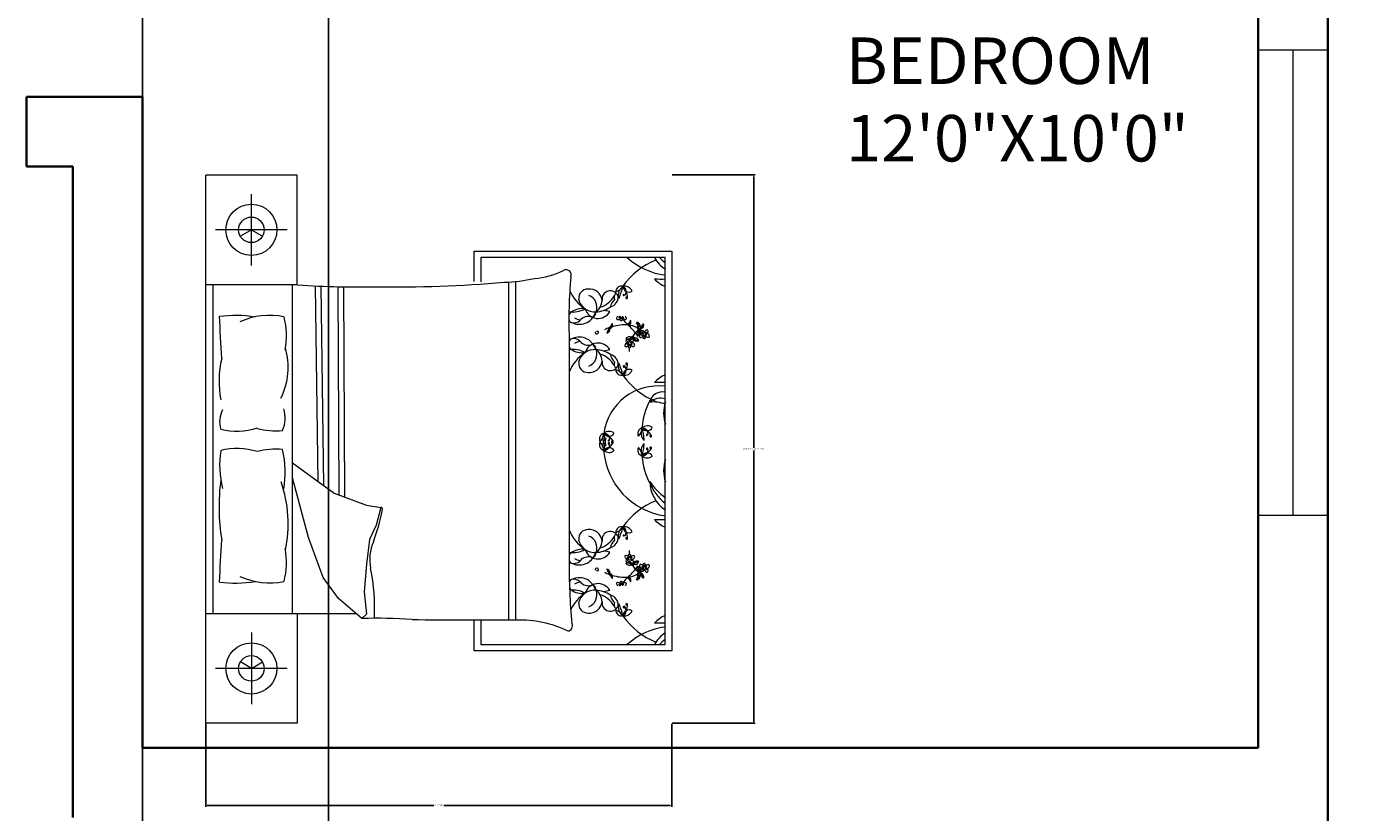
# Model space of a CAD drawing. Units: inches. Extents: x -43 to 1296, y -568 to 542.
# Tile 10 of 14: x 1016 to 1187, y -354 to -253. Entities that reach past the tile are written whole.
import ezdxf

# ---------------------------------------------------------------- set-up
doc = ezdxf.new("R2010")
doc.units = ezdxf.units.IN
doc.header["$MEASUREMENT"] = 0
for name, color, linetype, lineweight in [('A-ANNO-DIMS', 2, 'Continuous', 18), ('A-AREA-IDEN', 7, 'Continuous', 18), ('A-FURN', 8, 'Continuous', 13), ('A-GLAZ', 6, 'Continuous', 18), ('A-WALL', 7, 'Continuous', 35)]:
    doc.layers.add(name, color=color, linetype=linetype, lineweight=lineweight)
doc.styles.get("Standard").update_dxf_attribs({"font": 'arial.ttf'})
doc.dimstyles.get("Standard").update_dxf_attribs({"dimtxt": 0.18, "dimasz": 0.18, "dimexe": 0.18, "dimexo": 0.0625, "dimgap": 0.09, "dimtad": 0, "dimtih": 1, "dimtoh": 1, "dimdec": 0, "dimzin": 0, "dimdsep": 46, "dimlunit": 3, "dimtxsty": 'Standard', "dimcen": 0.09, "dimadec": 0, "dimazin": 0, "dimtfac": 1, "dimtdec": 0, "dimtofl": 0, "dimtmove": 0, "dimatfit": 3, "dimfxl": 1, "dimtolj": 1, "dimtzin": 0, "dimarcsym": 0})

# ---------------------------------------------------------------- blocks, each defined once
blk = doc.blocks.new('*D4')
at = {"layer": 'A-ANNO-DIMS', "color": 0, "lineweight": -2, "transparency": 16777216}
for p, q in [((1184.19, -3.76), (1201.25, -3.76)), ((1201.07, -3.94), (1201.07, -240.61)), ((1201.07, -483.58), (1201.07, -246.91)), ((1184.19, -483.76), (1201.25, -483.76))]:
    blk.add_line(p, q, dxfattribs=at)
at = {"layer": 'A-ANNO-DIMS', "color": 0, "transparency": 16777216}
for points in [[(1201.04, -3.94), (1201.1, -3.94), (1201.07, -3.76)], [(1201.04, -483.58), (1201.1, -483.58), (1201.07, -483.76)]]:
    blk.add_solid(points, dxfattribs=at)
at = {"layer": 'Defpoints', "color": 0, "transparency": 16777216}
for p in [(1184.13, -3.76), (1184.13, -483.76), (1201.07, -483.76)]:
    blk.add_point(p, dxfattribs=at)
at = {"layer": 'A-ANNO-DIMS', "color": 0, "transparency": 16777216, "insert": (1201.07, -243.76), "char_height": 6, "attachment_point": 5}
blk.add_mtext("\\A1;40'", dxfattribs=at)
blk = doc.blocks.new('BED-SUITE-71')
for p, q in [((0, 0), (0, 70.73)), ((5.89, 59.04), (5.89, 68.28)), ((10.52, 63.66), (1.27, 63.66)), ((34.67, 56.98), (34.67, 60.9)), ((34.67, 60.9), (60.15, 60.9)), ((35.49, 60.08), (35.49, 56.97)), ((59.33, 60.08), (35.49, 60.08)), ((59.33, 10.16), (59.33, 60.08)), ((60.15, 60.9), (60.15, 9.34)), ((0.91, 56.59), (0.91, 14.15)), ((11.18, 14.15), (11.18, 56.59)), ((14.12, 56.4), (14.47, 31.21)), ((39.09, 56.91), (39.09, 13.33)), ((39.97, 56.97), (39.97, 13.33)), ((14.84, 56.37), (15.21, 30.69)), ((17.07, 56.33), (17.18, 29.47)), ((17.8, 56.34), (17.91, 29.2)), ((52.16, 53.11), (51.36, 53.27)), ((46.92, 49.73), (46.92, 21.01)), ((52.16, 48.17), (51.36, 48.01)), ((11.18, 33.58), (16.57, 29.7)), ((13.28, 23.97), (11.18, 31.68)), ((16.57, 29.7), (20.73, 28.13)), ((20.73, 28.13), (22.59, 27.84)), ((22.59, 27.84), (22.01, 25.55)), ((15.14, 18.81), (13.28, 23.97)), ((22.01, 25.55), (21.15, 23.69)), ((21.15, 23.69), (20.73, 20.53)), ((52.16, 22.07), (51.36, 22.23)), ((20.73, 20.53), (20.44, 16.95)), ((17.15, 16.09), (15.14, 18.81)), ((52.16, 17.13), (51.36, 16.97)), ((20.15, 13.51), (17.15, 16.09)), ((20.44, 16.95), (20.73, 14.09)), ((0, 14.15), (19.41, 14.15)), ((20.73, 14.09), (20.15, 13.51)), ((34.67, 9.34), (34.67, 13.34)), ((35.49, 13.34), (35.49, 10.16)), ((5.89, 11.69), (5.89, 2.45)), ((60.15, 9.34), (34.67, 9.34)), ((35.49, 10.16), (59.33, 10.16)), ((10.52, 7.07), (1.27, 7.07))]:
    blk.add_line(p, q)
for points in [[(0, 56.59), (11.79, 56.59), (11.79, 70.73), (0, 70.73)], [(5.89, 63.66), (4.47, 62.83)], [(5.89, 63.66), (7.32, 62.83)], [(11.79, 14.15), (11.79, 0), (0, 0)], [(5.89, 7.07), (4.47, 7.9)], [(5.89, 7.07), (7.32, 7.9)]]:
    blk.add_lwpolyline(points)
for points in [[(38.53, 56.89, 0.056112), (42.42, 57.4, 0.095341), (46.17, 58.4)], [(1.76, 52.52, -0.074897), (6.38, 52.44, 0.472817)], [(6.64, 38.06, -0.14099), (1.93, 37.91, -0.235245)], [(6.64, 35.04, 0.14099), (1.93, 35.18, 0.235245)], [(1.76, 18.21, 0.074897), (6.38, 18.3, -0.472817)], [(26.63, 13.37, 0.001242), (40.05, 13.33, -0.127202), (46.74, 11.91)]]:
    blk.add_lwpolyline(points, format="xyb")
for centre, radius in [((5.89, 63.66), 3.3), ((5.89, 63.66), 1.65), ((56.62, 50.21), 0.18), ((54.73, 49.03), 0.18), ((54.73, 21.21), 0.18), ((56.62, 20.03), 0.18), ((5.89, 7.07), 3.3), ((5.89, 7.07), 1.65)]:
    blk.add_circle(centre, radius)
for centre, radius, start, end in [((60.58, 66.96), 9.24, 228.1144, 262.255), ((61.82, 62.33), 4.5, 209.8884, 236.5383), ((62.65, 63.95), 5.61, 223.5186, 233.6964), ((46.53, 57.86), 0.645, 336.5219, 123.8264), ((61.49, 51.16), 9.24, 111.4092, 145.6135), ((19.82, 183.39), 127.09, 266.1, 270.9282), ((24.44, 222.08), 165.79, 269.1145, 274.8735), ((115.71, 51.89), 68.83, 175.2402, 181.8035), ((53.69, 55.63), 0.766, 76.272, 177.0484), ((52.52, 57.2), 1.58, 284.7031, 328.6173), ((54.72, 55.19), 1.46, 125.7657, 194.5347), ((47.56, 57.77), 6.46, 332.8176, 347.4827), ((54.09, 55.37), 1.02, 20.9613, 102.2885), ((54.64, 56.4), 0.771, 181.7131, 301.5367), ((52.11, 54.84), 2.34, 2.0648, 41.1598), ((53.52, 55.71), 0.756, 316.2238, 62.3173), ((60.77, 59.81), 3.76, 221.0454, 247.4453), ((58.76, 70.09), 12.78, 266.3481, 272.5919), ((51.9, 57.95), 5.35, 203.6453, 236.3329), ((49.33, 54.83), 1.19, 88.9462, 185.5144), ((50.21, 55.2), 2.13, 193.079, 274.7067), ((49.5, 54.34), 1.69, 7.1143, 95.0551), ((48.86, 53.68), 1.64, 338.5779, 68.4181), ((49.88, 56.84), 3.34, 288.2955, 328.7386), ((52.22, 54.73), 1.06, 19.1312, 189.736), ((51.9, 54.99), 1.33, 285.6955, 4.031), ((53.66, 53.56), 1.41, 128.4175, 173.8338), ((53.37, 54.95), 0.651, 126.7319, 206.0245), ((53.95, 55.26), 0.0602, 20.2667, 316.2271), ((54.27, 54.93), 0.0557, 52.0591, 168.5166), ((54.33, 54.92), 0.115, 168.5166, 2.0648), ((47.44, 55.99), 2.93, 259.249, 301.1782), ((47.7, 52.36), 0.852, 127.675, 162.5814), ((48.2, 53.72), 2.25, 240.8249, 340.7178), ((48.71, 50.78), 2.73, 85.2696, 124.215), ((50.64, 53.99), 1.76, 196.8663, 330.0915), ((49.9, 52.88), 0.439, 254.8529, 12.6959), ((48.71, 50.78), 2.73, 53.6555, 57.2989), ((49.12, 54.64), 2.05, 305.9599, 357.6409), ((50.15, 56.87), 3.8, 273.4924, 303.7117), ((-671.38, 13.54), 674.27, 2.85022, 3.31479), ((8.24, 43.51), 9.12, 78.2417, 114.8684), ((0.94, 50), 9.48, 348.9631, 14.8961), ((47.7, 52.36), 0.852, 196.6343, 225.5483), ((47.53, 52.72), 1.06, 246.1646, 318.4347), ((48.61, 54.06), 2.03, 240.0851, 262.564), ((49.41, 51.05), 1.45, 74.8529, 138.4347), ((52.16, 51.3), 0.339, 265.7131, 351.6568), ((51.42, 52), 1.14, 313.6929, 321.7899), ((52.67, 51.22), 0.371, 115.5379, 168.6744), ((51.41, 51.75), 1.12, 329.344, 349.7412), ((54.13, 45.54), 5.86, 86.1723, 106.4158), ((50.52, 51.5), 1.99, 352.8698, 1.6736), ((53.16, 52.22), 0.139, 125.0752, 284.7644), ((53.38, 52.27), 0.3, 127.3642, 168.4363), ((53.14, 52.51), 0.433, 277.4968, 341.2737), ((53.48, 52.31), 0.172, 88.1325, 178.8919), ((53.83, 52.13), 0.372, 136.3462, 189.6513), ((53.62, 52.09), 0.155, 189.6513, 312.3208), ((53.66, 52.52), 0.18, 183.2768, 356.7232), ((54.22, 52.2), 0.59, 164.2829, 186.9148), ((53.52, 52.19), 0.295, 312.3208, 40.2111), ((54.15, 52.53), 0.419, 201.6382, 274.947), ((53.59, 51.95), 0.547, 42.3896, 66.5724), ((59.11, 56.28), 6.72, 217.9541, 226.8459), ((53.99, 52.27), 0.297, 10.9597, 52.2379), ((54.17, 52.25), 0.138, 274.947, 37.5263), ((54.64, 51.46), 0.144, 112.5583, 214.2343), ((54.54, 51.72), 0.339, 265.7131, 351.6568), ((54.24, 51.91), 0.593, 297.3659, 329.344), ((54.27, 48.45), 2.94, 60.7959, 85.244), ((48.02, 44.23), 9.66, 37.8256, 47.7588), ((53.8, 52.42), 1.14, 313.6929, 321.7899), ((55.05, 51.64), 0.371, 115.5379, 168.6744), ((53.79, 52.18), 1.12, 329.344, 349.7412), ((52.9, 51.92), 1.99, 352.8698, 1.6736), ((55.7, 51.52), 0.201, 33.0979, 123.1364), ((51.27, 48.68), 5.26, 31.1156, 34.8118), ((55.41, 51.17), 0.545, 2.3172, 70.5201), ((55.6, 51.29), 0.208, 315.7354, 31.1156), ((55.62, 51.23), 0.469, 352.6008, 57.1845), ((56.07, 51.34), 0.469, 252.8042, 349.6943), ((56.12, 51.38), 0.208, 248.2452, 323.6254), ((55.93, 51.5), 0.545, 291.7087, 3.0299), ((52.05, 54.37), 5.26, 323.6254, 327.3216), ((56.36, 51.37), 0.201, 325.6077, 55.6462), ((48.2, 47.57), 2.25, 19.2822, 119.1751), ((47.53, 48.57), 1.06, 41.5653, 113.8354), ((50.48, 50.45), 0.222, 169.5864, 349.5616), ((50.57, 50.44), 0.136, 349.5616, 167.2949), ((54.13, 45.54), 5.86, 110.1059, 116.9968), ((52.16, 50.36), 0.371, 129.5056, 182.6421), ((51.09, 51.22), 1.12, 308.4388, 328.836), ((50.9, 52.13), 1.99, 296.5064, 305.3102), ((50.88, 51.11), 1.14, 336.3901, 344.4871), ((52.12, 50.82), 0.144, 83.9457, 185.6216), ((51.54, 50.95), 0.593, 328.836, 0.8141), ((51.85, 50.78), 0.339, 306.5232, 32.4668), ((52.26, 51.04), 0.144, 112.5583, 214.2343), ((51.86, 51.49), 0.593, 297.3659, 329.344), ((54.46, 50.41), 0.821, 253.6301, 325.4631), ((54.69, 49.27), 0.581, 82.0748, 142.6895), ((54.62, 50.06), 0.597, 228.342, 274.9894), ((54.64, 49.97), 0.499, 273.8774, 357.1501), ((55.27, 49.07), 0.568, 121.9501, 165.2442), ((54.84, 50.32), 0.483, 262.0748, 308.2393), ((58.17, 48.15), 3.52, 156.1523, 156.9499), ((55.06, 49.41), 0.178, 44.3732, 121.9501), ((55.61, 49.82), 0.499, 181.4625, 249.4747), ((55.53, 50.22), 0.483, 215.1128, 261.2773), ((55.92, 50.19), 0.821, 197.889, 269.722), ((58.17, 48.15), 3.52, 130.182, 149.456), ((55.37, 49.17), 0.581, 20.6625, 81.2773), ((56.23, 50.16), 0.581, 139.3812, 199.9959), ((55.15, 50.58), 0.821, 310.9365, 22.7695), ((55.53, 50.53), 0.597, 285.6484, 332.2957), ((55.86, 51.04), 0.157, 135.7354, 318.1297), ((55.43, 50.85), 0.483, 319.3812, 5.5456), ((55.98, 51.04), 0.157, 68.2452, 250.6395), ((57.29, 48.08), 3.14, 111.7087, 116.2181), ((54.27, 48.45), 2.94, 47.5083, 55.9967), ((55.62, 50.5), 0.499, 331.1838, 51.6792), ((56.13, 49.9), 0.139, 125.0752, 284.7644), ((56.35, 49.96), 0.3, 93.635, 168.4363), ((56.31, 50.43), 0.176, 138.2946, 276.2474), ((56.11, 50.2), 0.433, 277.4968, 341.2737), ((56.37, 50.4), 0.246, 358.5719, 143.8954), ((56.45, 50), 0.172, 88.1325, 178.8919), ((56.52, 50.6), 0.248, 208.8493, 269.9355), ((56.31, 50.54), 0.283, 274.2123, 318.1587), ((56.8, 49.81), 0.372, 136.3462, 189.6513), ((56.59, 49.78), 0.155, 189.6513, 312.3208), ((57.19, 49.88), 0.59, 164.2829, 186.9148), ((57.17, 50.25), 0.568, 121.9501, 165.2442), ((56.49, 49.88), 0.295, 312.3208, 40.2111), ((57.12, 50.21), 0.419, 201.6382, 274.947), ((56.78, 50.47), 0.119, 262.868, 7.094), ((56.56, 49.64), 0.547, 42.3896, 66.5724), ((56.76, 50.57), 0.355, 278.5614, 22.5914), ((56.96, 49.96), 0.297, 10.9597, 118.7804), ((56.96, 50.58), 0.178, 44.3732, 121.9501), ((57.14, 49.93), 0.138, 274.947, 37.5263), ((1.63, 45.91), 9, 333.8761, 16.1746), ((47.7, 48.93), 0.852, 134.4517, 156.7144), ((47.7, 48.93), 0.852, 203.2856, 232.325), ((47.44, 45.3), 2.93, 58.8218, 100.2867), ((48.71, 50.51), 2.73, 235.785, 274.7304), ((48.61, 47.23), 2.03, 97.436, 119.9149), ((50.21, 46.08), 2.13, 85.2933, 166.921), ((49.41, 50.23), 1.45, 221.5653, 285.1471), ((50.64, 47.29), 1.76, 29.9085, 163.1337), ((48.86, 47.61), 1.64, 291.5819, 21.4221), ((49.9, 48.41), 0.439, 347.3041, 105.1471), ((48.71, 50.51), 2.73, 302.7011, 306.3445), ((49.12, 46.65), 2.05, 2.3591, 54.0401), ((50.15, 44.42), 3.8, 56.2883, 86.5076), ((54.23, 48.72), 0.139, 125.0752, 284.7644), ((54.45, 48.78), 0.3, 93.635, 168.4363), ((54.41, 49.25), 0.176, 138.2946, 276.2474), ((54.21, 49.02), 0.433, 277.4968, 341.2737), ((54.48, 49.23), 0.246, 358.5719, 143.8954), ((54.56, 48.82), 0.172, 88.1325, 178.8919), ((54.62, 49.42), 0.248, 208.8493, 269.9355), ((54.41, 49.36), 0.283, 274.2123, 318.1587), ((54.9, 48.63), 0.372, 136.3462, 189.6513), ((54.69, 48.6), 0.155, 189.6513, 312.3208), ((58.17, 48.15), 3.52, 175.2415, 182.8929), ((55.29, 48.7), 0.59, 164.2829, 186.9148), ((54.59, 48.7), 0.295, 312.3208, 40.2111), ((55.22, 49.03), 0.419, 201.6382, 274.947), ((54.88, 49.29), 0.119, 262.868, 7.094), ((54.66, 48.46), 0.547, 42.3896, 66.5724), ((54.86, 49.39), 0.355, 278.5614, 22.5914), ((55.06, 48.78), 0.297, 10.9597, 118.7804), ((55.24, 48.75), 0.138, 274.947, 37.5263), ((55.66, 49.91), 0.597, 248.3627, 295.0101), ((14.14, 44.13), 12.43, 166.3427, 191.1841), ((51.9, 43.33), 5.35, 123.6671, 158.5059), ((49.33, 46.45), 1.19, 174.4856, 271.0538), ((49.5, 46.94), 1.69, 264.9449, 352.8857), ((49.88, 44.45), 3.34, 31.2614, 71.7045), ((52.22, 46.55), 1.06, 170.264, 340.8688), ((53.66, 47.73), 1.41, 186.1662, 231.5825), ((51.9, 46.3), 1.33, 355.969, 74.3045), ((53.37, 46.33), 0.651, 153.9755, 233.2681), ((54.72, 46.09), 1.46, 165.4653, 234.2343), ((47.56, 43.51), 6.46, 12.5173, 27.1824), ((52.11, 46.45), 2.34, 318.8402, 357.9352), ((53.99, 46.03), 0.0999, 43.7762, 339.7183), ((54.33, 46.37), 0.115, 357.9352, 191.4834), ((54.27, 46.35), 0.0557, 191.4834, 307.9409), ((53.69, 45.65), 0.766, 182.9516, 283.728), ((52.52, 44.09), 1.58, 31.3827, 75.2969), ((53.52, 45.58), 0.756, 297.6827, 43.7762), ((54.64, 44.89), 0.771, 58.4633, 178.2869), ((54.09, 45.91), 1.02, 257.7115, 339.0387), ((61.49, 50.13), 9.24, 214.3865, 248.5908), ((60.77, 41.48), 3.76, 112.5547, 138.9546), ((58.45, 36.38), 7.15, 82.8636, 171.8197), ((58.94, 41.1), 1.66, 76.3898, 169.0739), ((58.76, 31.19), 12.78, 87.4081, 93.6519), ((65.53, 37.39), 9.24, 152.5854, 175.5377), ((58.72, 39.85), 2.1, 72.8609, 131.9049), ((57.79, 37.31), 4.14, 68.117, 96.6195), ((64.19, 39.97), 5.08, 162.9798, 196.4569), ((5.29, 38.88), 3.5, 153.3437, 196.1026), ((6.51, 39.36), 3.75, 335.0183, 18.5407), ((9.01, 46.39), 8.67, 254.1707, 275.9871), ((52.06, 36.64), 1.02, 50.8855, 132.2127), ((56.53, 37.37), 0.766, 106.1963, 206.9726), ((54.74, 38.15), 1.58, 314.6273, 358.5415), ((57.65, 37.51), 1.46, 155.6899, 224.4589), ((57.01, 37.35), 1.02, 50.8855, 132.2127), ((56.97, 38.51), 0.771, 211.6373, 331.4609), ((55.56, 35.9), 2.34, 31.989, 71.0841), ((50.15, 36.17), 6.46, 2.7418, 17.407), ((56.35, 37.35), 0.756, 346.148, 92.2415), ((66.81, 37.96), 7.51, 174.3643, 175.6213), ((71.95, 34), 13.42, 160.0972, 160.2783), ((51.58, 36.66), 0.766, 106.1963, 206.9726), ((51.58, 35.93), 0.766, 153.0274, 253.8037), ((49.79, 37.44), 1.58, 314.6273, 358.5415), ((49.79, 35.16), 1.58, 1.4585, 45.3727), ((52.7, 36.8), 1.46, 155.6899, 224.4589), ((52.7, 35.8), 1.46, 135.5411, 204.3101), ((52.03, 37.8), 0.771, 211.6373, 331.4609), ((51.4, 36.64), 0.756, 346.148, 92.2415), ((50.61, 35.19), 2.34, 31.989, 71.0841), ((45.2, 35.47), 6.46, 2.7418, 17.407), ((45.2, 37.13), 6.46, 342.593, 357.2582), ((50.61, 37.41), 2.34, 288.9159, 328.011), ((51.4, 35.95), 0.756, 267.7585, 13.852), ((52, 36.48), 0.0602, 50.1909, 346.0209), ((52.04, 36.11), 0.0999, 13.852, 309.9245), ((52.5, 36.37), 0.115, 198.4408, 31.989), ((52.44, 36.35), 0.0557, 81.9833, 198.4408), ((52.5, 36.23), 0.115, 328.011, 161.5592), ((52.44, 36.25), 0.0557, 161.5592, 278.0167), ((57.65, 35.09), 1.46, 135.5411, 204.3101), ((50.15, 36.42), 6.46, 342.593, 357.2582), ((56.94, 37.19), 0.0602, 50.1909, 346.0209), ((57.39, 37.05), 0.0557, 81.9833, 198.4408), ((57.44, 37.07), 0.115, 198.4408, 31.989), ((14.39, 33.32), 12.6, 171.5249, 193.96), ((9.01, 26.7), 8.67, 84.0129, 105.8293), ((-2.21, 32.38), 12.47, 349.8617, 13.6238), ((52.03, 34.79), 0.771, 28.5391, 148.3627), ((52.06, 35.96), 1.02, 227.7873, 309.1145), ((60.58, 35.92), 9.24, 184.4623, 262.255), ((56.53, 35.23), 0.766, 153.0274, 253.8037), ((54.74, 34.45), 1.58, 1.4585, 45.3727), ((55.56, 36.7), 2.34, 288.9159, 328.011), ((56.35, 35.25), 0.756, 267.7585, 13.852), ((56.97, 34.09), 0.771, 28.5391, 148.3627), ((57.01, 35.25), 1.02, 227.7873, 309.1145), ((65.53, 35.21), 9.24, 184.4623, 207.4146), ((56.98, 35.4), 0.0999, 13.852, 309.9245), ((57.39, 35.54), 0.0557, 161.5592, 278.0167), ((57.44, 35.52), 0.115, 328.011, 161.5592), ((64.19, 32.63), 5.08, 163.5431, 197.0202), ((66.81, 34.64), 7.51, 184.3787, 185.6357), ((71.95, 38.59), 13.42, 199.7217, 199.9028), ((27.36, 27.9), 25.65, 172.2196, 189.497), ((-5.8, 25.72), 16.44, 348.0397, 19.2615), ((61.82, 31.28), 4.5, 181.272, 236.5383), ((64.23, 35.85), 8.34, 214.0123, 234.053), ((62.65, 32.9), 5.61, 197.8504, 233.6964), ((-4.14, 32.75), 27.43, 340.1194, 349.3383), ((22.64, 27.68), 0.171, 358.8623, 109.7536), ((61.49, 20.11), 9.24, 111.4092, 145.6135), ((58.76, 39.05), 12.78, 266.3481, 272.5919), ((60.77, 28.76), 3.76, 221.0454, 247.4453), ((51.9, 26.91), 5.35, 201.4941, 236.3329), ((49.33, 23.79), 1.19, 88.9462, 185.5144), ((49.5, 23.3), 1.69, 7.1143, 95.0551), ((48.86, 22.63), 1.64, 338.5779, 68.4181), ((49.88, 25.79), 3.34, 288.2955, 328.7386), ((52.22, 23.69), 1.06, 19.1312, 189.736), ((51.9, 23.94), 1.33, 285.6955, 4.031), ((53.37, 23.91), 0.651, 126.7319, 206.0245), ((53.69, 24.59), 0.766, 76.272, 177.0484), ((52.52, 26.15), 1.58, 284.7031, 328.6173), ((54.72, 24.15), 1.46, 125.7657, 194.5347), ((47.56, 26.73), 6.46, 332.8176, 347.4827), ((54.09, 24.33), 1.02, 20.9613, 102.2885), ((53.52, 24.66), 0.756, 316.2238, 62.3173), ((52.11, 23.79), 2.34, 2.0648, 41.1598), ((54.64, 25.35), 0.771, 181.7131, 301.5367), ((53.95, 24.22), 0.0602, 20.2667, 316.2271), ((54.27, 23.88), 0.0557, 52.0591, 168.5166), ((-671.38, 57.2), 674.27, 356.68521, 357.14978), ((0.94, 20.73), 9.48, 345.1039, 11.0369), ((26.92, 21.1), 5.76, 156.2616, 191.3392), ((47.44, 24.94), 2.93, 259.7133, 301.1782), ((48.71, 19.73), 2.73, 85.2696, 124.215), ((50.21, 24.15), 2.13, 193.079, 274.7067), ((50.64, 22.95), 1.76, 196.8663, 330.0915), ((49.12, 23.59), 2.05, 305.9599, 357.6409), ((50.15, 25.82), 3.8, 273.4924, 303.7117), ((53.66, 22.51), 1.41, 128.4175, 173.8338), ((54.33, 23.87), 0.115, 168.5166, 2.0648), ((58.17, 22.09), 3.52, 177.1071, 184.7585), ((120.54, 20.16), 73.63, 179.3433, 185.6887), ((47.7, 21.31), 0.852, 127.675, 156.7144), ((47.7, 21.31), 0.852, 203.229, 225.5483), ((48.2, 22.67), 2.25, 240.8249, 340.7178), ((47.53, 21.67), 1.06, 246.1646, 318.4347), ((48.61, 23.01), 2.03, 240.0851, 262.564), ((49.41, 20.01), 1.45, 74.8529, 138.4347), ((49.9, 21.83), 0.439, 254.8529, 12.6959), ((48.71, 19.73), 2.73, 53.6555, 57.2989), ((54.23, 21.52), 0.139, 75.2356, 234.9248), ((54.45, 21.46), 0.3, 191.5637, 266.365), ((54.41, 20.99), 0.176, 83.7526, 221.7054), ((54.62, 20.18), 0.597, 85.0106, 131.658), ((54.46, 19.83), 0.821, 34.5369, 106.3699), ((54.69, 20.97), 0.581, 217.3105, 277.9252), ((54.21, 21.22), 0.433, 18.7263, 82.5032), ((54.48, 21.01), 0.246, 216.1046, 1.4281), ((54.56, 21.42), 0.172, 181.1081, 271.8675), ((54.62, 20.82), 0.248, 90.0645, 151.1507), ((54.41, 20.88), 0.283, 41.8413, 85.7877), ((54.69, 21.64), 0.155, 47.6792, 170.3487), ((54.9, 21.61), 0.372, 170.3487, 223.6538), ((54.64, 20.27), 0.499, 2.8499, 86.1226), ((55.29, 21.53), 0.59, 173.0852, 195.7171), ((55.27, 21.16), 0.568, 194.7558, 238.0499), ((54.59, 21.54), 0.295, 319.7889, 47.6792), ((55.22, 21.21), 0.419, 85.053, 158.3618), ((54.88, 20.95), 0.119, 352.906, 97.132), ((54.66, 21.78), 0.547, 293.4276, 317.6104), ((55.06, 21.46), 0.297, 241.2196, 349.0403), ((54.86, 20.85), 0.355, 337.4086, 81.4386), ((58.17, 22.09), 3.52, 203.0501, 203.8477), ((55.06, 20.83), 0.178, 238.0499, 315.6268), ((55.61, 20.41), 0.499, 110.5253, 178.5375), ((55.92, 20.05), 0.821, 90.278, 162.111), ((55.53, 20.02), 0.483, 98.7227, 144.8872), ((55.24, 21.49), 0.138, 322.4737, 85.053), ((55.66, 20.33), 0.597, 64.9899, 111.6373), ((55.37, 21.07), 0.581, 278.7227, 339.3375), ((56.59, 20.46), 0.155, 47.6792, 170.3487), ((56.49, 20.36), 0.295, 319.7889, 47.6792), ((8.24, 27.22), 9.12, 245.1316, 281.7583), ((-4.9, 14.72), 26.7, 357.4519, 11.3392), ((50.48, 19.79), 0.222, 10.4384, 190.4136), ((50.57, 19.8), 0.136, 192.7051, 10.4384), ((54.13, 24.7), 5.86, 243.0032, 249.8941), ((51.09, 19.02), 1.12, 31.164, 51.5612), ((52.16, 19.88), 0.371, 177.3579, 230.4944), ((50.9, 18.11), 1.99, 54.6898, 63.4936), ((50.88, 19.13), 1.14, 15.5129, 23.6099), ((52.12, 19.42), 0.144, 174.3784, 276.0543), ((51.85, 19.46), 0.339, 327.5332, 53.4768), ((51.54, 19.29), 0.593, 359.1859, 31.164), ((52.26, 19.2), 0.144, 145.7657, 247.4417), ((52.16, 18.94), 0.339, 8.3432, 94.2869), ((51.86, 18.75), 0.593, 30.656, 62.6341), ((51.42, 18.24), 1.14, 38.2101, 46.3071), ((52.67, 19.02), 0.371, 191.3256, 244.4621), ((51.41, 18.49), 1.12, 10.2588, 30.656), ((54.13, 24.7), 5.86, 253.5842, 273.8277), ((50.52, 18.74), 1.99, 358.3264, 7.1302), ((59.11, 13.96), 6.72, 133.1541, 142.0459), ((54.64, 18.78), 0.144, 145.7657, 247.4417), ((48.02, 26.01), 9.66, 312.2412, 322.1744), ((54.27, 21.79), 2.94, 274.756, 299.2041), ((54.54, 18.52), 0.339, 8.3432, 94.2869), ((54.24, 18.33), 0.593, 30.656, 62.6341), ((54.84, 19.92), 0.483, 51.7607, 97.9252), ((58.17, 22.09), 3.52, 210.544, 229.818), ((55.41, 19.07), 0.545, 289.4799, 357.6828), ((51.27, 21.56), 5.26, 325.1882, 328.8844), ((56.23, 20.08), 0.581, 160.0041, 220.6188), ((55.15, 19.66), 0.821, 337.2305, 49.0635), ((55.53, 19.71), 0.597, 27.7043, 74.3516), ((55.86, 19.2), 0.157, 41.8703, 224.2646), ((55.6, 18.95), 0.208, 328.8844, 44.2646), ((55.43, 19.39), 0.483, 354.4544, 40.6188), ((55.98, 19.2), 0.157, 109.3605, 291.7548), ((55.62, 19.01), 0.469, 302.8155, 7.3992), ((57.29, 22.16), 3.14, 243.7819, 248.2913), ((54.27, 21.79), 2.94, 304.0033, 312.4917), ((55.62, 19.74), 0.499, 308.3208, 28.8162), ((56.07, 18.9), 0.469, 10.3057, 107.1958), ((56.13, 20.34), 0.139, 75.2356, 234.9248), ((56.12, 18.86), 0.208, 36.3746, 111.7548), ((56.35, 20.28), 0.3, 191.5637, 266.365), ((56.31, 19.81), 0.176, 83.7526, 221.7054), ((55.93, 18.74), 0.545, 356.9701, 68.2913), ((56.11, 20.04), 0.433, 18.7263, 82.5032), ((56.37, 19.84), 0.246, 216.1046, 1.4281), ((56.45, 20.24), 0.172, 181.1081, 271.8675), ((52.05, 15.87), 5.26, 32.6784, 36.3746), ((56.52, 19.64), 0.248, 90.0645, 151.1507), ((56.31, 19.7), 0.283, 41.8413, 85.7877), ((56.8, 20.43), 0.372, 170.3487, 223.6538), ((56.36, 18.87), 0.201, 304.3538, 34.3923), ((57.19, 20.36), 0.59, 173.0852, 195.7171), ((57.17, 19.99), 0.568, 194.7558, 238.0499), ((57.12, 20.03), 0.419, 85.053, 158.3618), ((56.78, 19.77), 0.119, 352.906, 97.132), ((56.56, 20.6), 0.547, 293.4276, 317.6104), ((56.96, 20.28), 0.297, 241.2196, 349.0403), ((56.76, 19.67), 0.355, 337.4086, 81.4386), ((56.96, 19.66), 0.178, 238.0499, 315.6268), ((57.14, 20.31), 0.138, 322.4737, 85.053), ((47.7, 17.88), 0.852, 134.4517, 153.558), ((47.7, 17.88), 0.852, 210.0293, 232.325), ((47.44, 14.25), 2.93, 58.8218, 99.1554), ((48.2, 16.52), 2.25, 19.2822, 119.1751), ((47.53, 17.52), 1.06, 41.5653, 113.8354), ((48.71, 19.46), 2.73, 235.785, 274.7304), ((48.61, 16.18), 2.03, 97.436, 119.9149), ((50.21, 15.04), 2.13, 85.2933, 166.921), ((49.41, 19.19), 1.45, 221.5653, 285.1471), ((50.64, 16.25), 1.76, 29.9085, 163.1337), ((48.86, 16.56), 1.64, 291.5819, 21.4221), ((49.9, 17.36), 0.439, 347.3041, 105.1471), ((48.71, 19.46), 2.73, 302.7011, 306.3445), ((49.12, 15.6), 2.05, 2.3591, 54.0401), ((50.15, 13.37), 3.8, 56.2883, 86.5076), ((53.16, 18.02), 0.139, 75.2356, 234.9248), ((53.38, 17.97), 0.3, 191.5637, 232.6358), ((53.14, 17.73), 0.433, 18.7263, 82.5032), ((53.48, 17.93), 0.172, 181.1081, 271.8675), ((53.62, 18.15), 0.155, 47.6792, 170.3487), ((53.83, 18.11), 0.372, 170.3487, 223.6538), ((53.66, 17.72), 0.18, 3.2768, 176.7232), ((54.22, 18.04), 0.59, 173.0852, 195.7171), ((53.52, 18.05), 0.295, 319.7889, 47.6792), ((54.15, 17.71), 0.419, 85.053, 158.3618), ((53.59, 18.29), 0.547, 293.4276, 317.6104), ((53.99, 17.97), 0.297, 307.7621, 349.0403), ((54.17, 17.99), 0.138, 322.4737, 85.053), ((53.8, 17.82), 1.14, 38.2101, 46.3071), ((55.05, 18.6), 0.371, 191.3256, 244.4621), ((53.79, 18.06), 1.12, 10.2588, 30.656), ((52.9, 18.32), 1.99, 358.3264, 7.1302), ((55.7, 18.72), 0.201, 236.8636, 326.9021), ((51.9, 12.29), 5.35, 123.6671, 153.2997), ((49.33, 15.41), 1.19, 174.4856, 271.0538), ((49.5, 15.9), 1.69, 264.9449, 352.8857), ((49.88, 13.4), 3.34, 31.2614, 71.7045), ((52.22, 15.51), 1.06, 170.264, 340.8688), ((51.9, 15.25), 1.33, 355.969, 74.3045), ((53.66, 16.68), 1.41, 186.1662, 231.5825), ((53.37, 15.29), 0.651, 153.9755, 233.2681), ((54.72, 15.05), 1.46, 165.4653, 234.2343), ((47.56, 12.46), 6.46, 12.5173, 27.1824), ((54.33, 15.32), 0.115, 357.9352, 191.4834), ((52.52, 13.04), 1.58, 31.3827, 75.2969), ((53.69, 14.61), 0.766, 182.9516, 283.728), ((52.11, 15.4), 2.34, 318.8402, 357.9352), ((53.52, 14.53), 0.756, 297.6827, 43.7762), ((54.64, 13.84), 0.771, 58.4633, 178.2869), ((54.09, 14.87), 1.02, 257.7115, 339.0387), ((61.49, 19.08), 9.24, 214.3865, 248.5908), ((53.99, 14.99), 0.0999, 43.7762, 339.7183), ((54.27, 15.31), 0.0557, 191.4834, 307.9409), ((60.77, 10.43), 3.76, 112.5547, 138.9546), ((21.91, -51.34), 64.88, 85.8294, 91.553), ((46.69, 12.56), 0.653, 273.98, 27.3412), ((60.58, 3.28), 9.24, 97.745, 131.8856), ((58.76, 0.15), 12.78, 87.4081, 93.6519), ((61.82, 7.91), 4.5, 123.4617, 150.1116), ((62.65, 6.29), 5.61, 126.3036, 136.4814)]:
    blk.add_arc(centre, radius, start, end)
blk = doc.blocks.new('WIN-60x9')
for p, q in [((0, 60), (0, 0)), ((9, 60), (0, 60)), ((4.5, 60), (4.5, 0)), ((9, 0), (9, 60)), ((0, 0), (9, 0))]:
    blk.add_line(p, q)
blk = doc.blocks.new('*D40')
at = {"layer": 'A-ANNO-DIMS', "color": 0, "lineweight": -2, "transparency": 16777216}
for p, q in [((1099.5, -271.85), (1110.22, -271.85)), ((1110.04, -272.03), (1110.04, -307.04)), ((1110.04, -342.41), (1110.04, -307.4)), ((1099.5, -342.59), (1110.22, -342.59))]:
    blk.add_line(p, q, dxfattribs=at)
at = {"layer": 'A-ANNO-DIMS', "color": 0, "transparency": 16777216}
for points in [[(1110.01, -272.03), (1110.07, -272.03), (1110.04, -271.85)], [(1110.01, -342.41), (1110.07, -342.41), (1110.04, -342.59)]]:
    blk.add_solid(points, dxfattribs=at)
at = {"layer": 'Defpoints', "color": 0, "transparency": 16777216}
for p in [(1099.43, -271.85), (1110.04, -271.85), (1099.43, -342.59)]:
    blk.add_point(p, dxfattribs=at)
at = {"layer": 'A-ANNO-DIMS', "color": 0, "transparency": 16777216, "insert": (1110.04, -307.22), "char_height": 0.18, "attachment_point": 5}
blk.add_mtext('\\A1;BED SET 5\'-10 1/2" TYP.', dxfattribs=at)
blk = doc.blocks.new('*D41')
at = {"layer": 'A-ANNO-DIMS', "color": 0, "lineweight": -2, "transparency": 16777216}
for p, q in [((1039.28, -342.65), (1039.28, -353.38)), ((1099.43, -342.65), (1099.43, -353.38)), ((1039.46, -353.2), (1068.72, -353.2)), ((1099.25, -353.2), (1070, -353.2))]:
    blk.add_line(p, q, dxfattribs=at)
at = {"layer": 'A-ANNO-DIMS', "color": 0, "transparency": 16777216}
for points in [[(1039.46, -353.17), (1039.46, -353.23), (1039.28, -353.2)], [(1099.25, -353.17), (1099.25, -353.23), (1099.43, -353.2)]]:
    blk.add_solid(points, dxfattribs=at)
at = {"layer": 'Defpoints', "color": 0, "transparency": 16777216}
for p in [(1039.28, -342.59), (1099.43, -342.59), (1099.43, -353.2)]:
    blk.add_point(p, dxfattribs=at)
at = {"layer": 'A-ANNO-DIMS', "color": 0, "transparency": 16777216, "insert": (1069.36, -353.2), "char_height": 0.18, "attachment_point": 5}
blk.add_mtext('\\A1;5\'-0" TYP.', dxfattribs=at)
blk = doc.blocks.new('*D83')
at = {"layer": 'A-ANNO-DIMS', "color": 0, "lineweight": -2, "transparency": 16777216}
for p, q in [((1031.13, -225.82), (1031.13, -532.44)), ((1055.13, -225.82), (1055.13, -532.44)), ((1031.31, -532.26), (1042.8, -532.26)), ((1054.95, -532.26), (1043.46, -532.26))]:
    blk.add_line(p, q, dxfattribs=at)
at = {"layer": 'A-ANNO-DIMS', "color": 0, "transparency": 16777216}
for points in [[(1031.31, -532.23), (1031.31, -532.29), (1031.13, -532.26)], [(1054.95, -532.23), (1054.95, -532.29), (1055.13, -532.26)]]:
    blk.add_solid(points, dxfattribs=at)
at = {"layer": 'Defpoints', "color": 0, "transparency": 16777216}
for p in [(1031.13, -225.76), (1055.13, -225.76), (1055.13, -532.26)]:
    blk.add_point(p, dxfattribs=at)
at = {"layer": 'A-ANNO-DIMS', "color": 0, "transparency": 16777216, "insert": (1043.13, -532.26), "char_height": 0.18, "attachment_point": 5}
blk.add_mtext('\\A1;2\'-0"', dxfattribs=at)

msp = doc.modelspace()

# ---------------------------------------------------------------- linework, layer by layer
at = {"layer": 'A-WALL'}
for p, q in [((1184.13, -3.76), (1184.13, -483.76)), ((1175.13, -225.76), (1175.13, -345.76)), ((1016.13, -261.76), (1031.13, -261.76)), ((1016.13, -261.76), (1016.13, -270.76)), ((1031.13, -261.76), (1031.13, -345.76)), ((1016.13, -270.76), (1022.13, -270.76)), ((1022.13, -270.76), (1022.13, -354.76)), ((1031.13, -345.76), (1175.13, -345.76))]:
    msp.add_line(p, q, dxfattribs=at)

# ---------------------------------------------------------------- block references
at = {"layer": 'A-FURN'}
msp.add_blockref('BED-SUITE-71', (1039.28, -342.59), dxfattribs=at)
at = {"layer": 'A-GLAZ'}
msp.add_blockref('WIN-60x9', (1175.13, -315.76), dxfattribs=at)

# ---------------------------------------------------------------- texts
at = {"layer": 'A-AREA-IDEN', "insert": (1121.93, -254.11), "char_height": 6, "attachment_point": 1}
msp.add_mtext('BEDROOM\\P12\'0"X10\'0"', dxfattribs=at)

# ---------------------------------------------------------------- dimensions: what is measured, and where the dimension line sits
at = {"layer": 'A-ANNO-DIMS'}
dim = msp.add_linear_dim(base=(1201.07, -483.76), p1=(1184.13, -3.76), p2=(1184.13, -483.76), angle=90, dimstyle='Standard', override={"dimtxt": 6, "dimclrd": 0, "dimclre": 0, "dimclrt": 0}, dxfattribs=at)
dim.commit()
dim.dimension.update_dxf_attribs({"geometry": '*D4', "text_midpoint": (1201.07, -243.76)})
dim = msp.add_linear_dim(base=(1055.13, -532.26), p1=(1031.13, -225.76), p2=(1055.13, -225.76), dimstyle='Standard', override={"dimdec": 1, "dimlfac": 1, "dimrnd": 0, "dimzin": 1, "dimdsep": 46, "dimlunit": 4, "dimfrac": 2}, dxfattribs=at)
dim.commit()
dim.dimension.update_dxf_attribs({"geometry": '*D83', "text_midpoint": (1043.13, -532.26)})
dim = msp.add_linear_dim(base=(1110.04, -271.85), p1=(1099.43, -342.59), p2=(1099.43, -271.85), angle=90, text='BED SET <> TYP.', dimstyle='Standard', override={"dimdec": 1, "dimlfac": 1, "dimrnd": 0, "dimzin": 1, "dimdsep": 46, "dimlunit": 4, "dimfrac": 2}, dxfattribs=at)
dim.commit()
dim.dimension.update_dxf_attribs({"geometry": '*D40', "text_midpoint": (1110.04, -307.22)})
dim = msp.add_linear_dim(base=(1099.4337, -353.1967), p1=(1039.2804, -342.5868), p2=(1099.4337, -342.5868), text='<> TYP.', dimstyle='Standard', override={"dimdec": 1, "dimlfac": 1, "dimrnd": 0, "dimzin": 1, "dimdsep": 46, "dimlunit": 4, "dimfrac": 2}, dxfattribs=at)
dim.commit()
dim.dimension.update_dxf_attribs({"geometry": '*D41', "text_midpoint": (1069.3571, -353.1967)})

doc.saveas('drawing.dxf')
